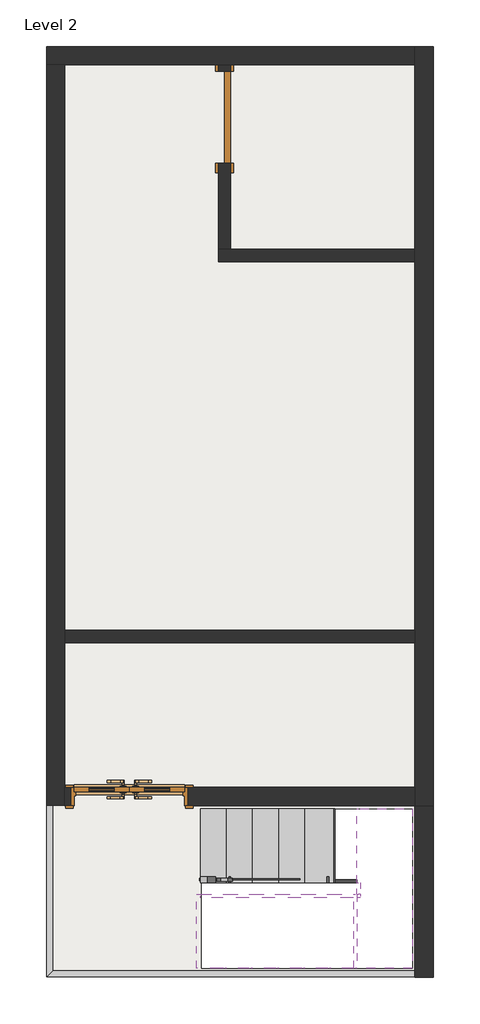
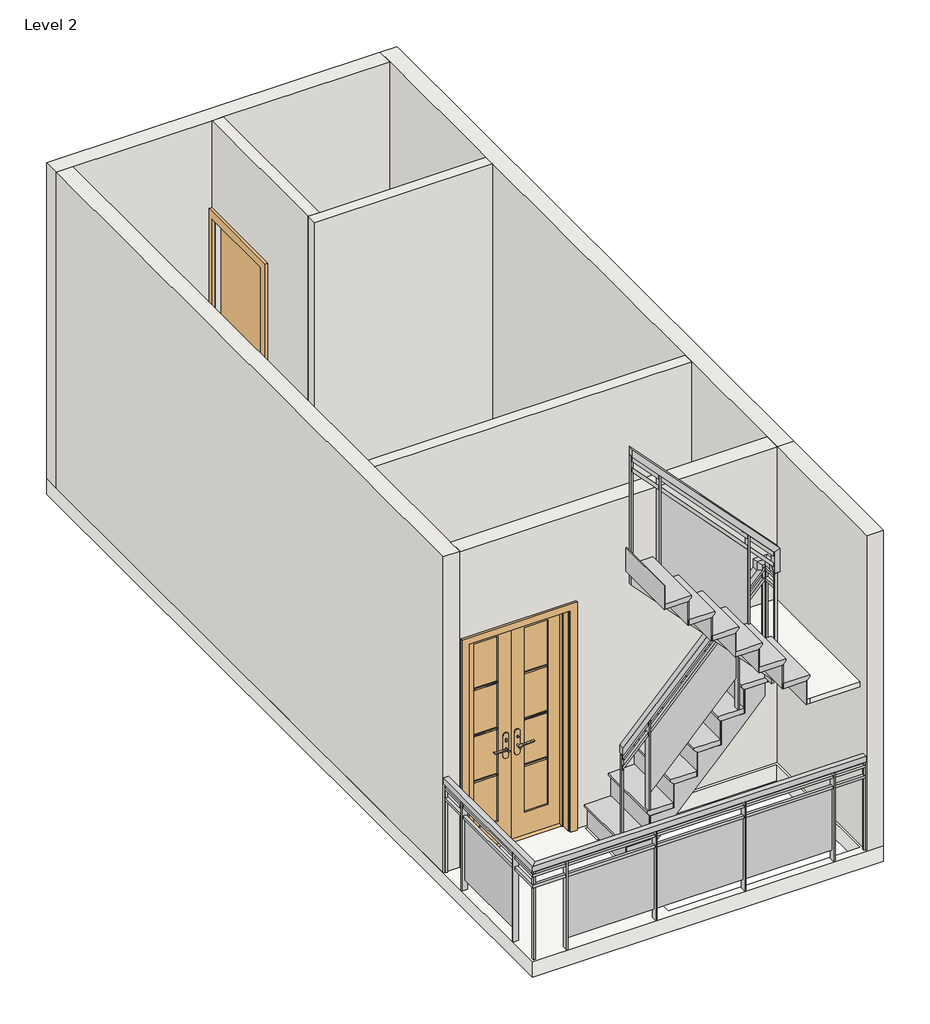
# One storey: 8 walls, 3 members, 2 doors, 2 railings, 2 slabs, 2 stair flights.
"""IFC4 building model written with IfcOpenShell, lengths in millimetres."""

from ifc_helpers import new_model, si_unit, frame, origin, place, context, project, spatial, polyline, outline, extrude, faceted_brep, transform, mapped, element, save
from components import door_665efd91, single_flush_2_5_aa9e95e7, non_monolithic_landing_3bfbdf2e, stair_flight_d5a7a9e1, stair_flight_0dc73603

model = new_model("IFC4")

# Units and contexts
model_context = context("Model", 3, world=origin())
ifc_project = project(units=[si_unit("LENGTHUNIT", "METRE", prefix="MILLI")], contexts=[model_context])

# Site, building, storey
site = spatial("IfcSite", under=ifc_project)
building = spatial("IfcBuilding", under=site)
storey = spatial("IfcBuildingStorey", under=building, Name="Level 2", Elevation=3200.4)

# Doors
placement = place(None, origin())
door_shape = door_665efd91(model_context)
element("IfcDoor", 1, ObjectType="Door-Exterior-Double-Full Glass-Wood_Clad : 60\" x 84\"", at=placement, inside=storey, context=model_context, shape_type="MappedRepresentation", body=[
    mapped(door_shape, transform((-5617.280937, -3133.7029636, 3200.4), x_axis=(1.0, 0.0, 0.0), y_axis=(0.0, 1.0, 0.0), z_axis=(0.0, 0.0, 1.0))),
])
single_flush_2_5_shape = single_flush_2_5_aa9e95e7(model_context)
element("IfcDoor", 2, ObjectType="Single-Flush : 2.5'", at=placement, inside=storey, context=model_context, shape_type="MappedRepresentation", body=[
    mapped(single_flush_2_5_shape, transform((-4829.880937, 2480.8335625, 3200.4), x_axis=(0.0, 1.0, 0.0), y_axis=(-1.0, 0.0, 0.0), z_axis=(0.0, 0.0, 1.0))),
])

# Members
element("IfcMember", 3, ObjectType="Carriage - 2\" Width", at=placement, inside=storey, context=model_context, shape_type="Brep", body=[
    faceted_brep([(-4996.3909298, -3822.6779636, 3200.4), (-4861.0694778, -3822.6779636, 3200.4), (-4861.0694778, -3848.0779636, 3200.4), (-4996.3909298, -3848.0779636, 3200.4), (-3732.7409298, -3822.6779636, 4395.1008155), (-3732.7409298, -3848.0779636, 4395.1008155), (-3916.8909298, -3848.0779636, 4200.1184625), (-4132.7909298, -3848.0779636, 3971.5184625), (-4348.6909298, -3848.0779636, 3742.9184625), (-4564.5909298, -3848.0779636, 3514.3184625), (-4780.4909298, -3848.0779636, 3285.7184625), (-3732.7409298, -3822.6779636, 4521.2), (-4996.3909298, -3822.6779636, 3378.2), (-4780.4909298, -3822.6779636, 3378.2), (-4780.4909298, -3822.6779636, 3606.8), (-4564.5909298, -3822.6779636, 3606.8), (-4564.5909298, -3822.6779636, 3835.4), (-4348.6909298, -3822.6779636, 3835.4), (-4348.6909298, -3822.6779636, 4064.0), (-4132.7909298, -3822.6779636, 4064.0), (-4132.7909298, -3822.6779636, 4292.6), (-3916.8909298, -3822.6779636, 4292.6), (-3916.8909298, -3822.6779636, 4521.2), (-3916.8909298, -3848.0779636, 4521.2), (-3732.7409298, -3848.0779636, 4521.2), (-3916.8909298, -3848.0779636, 4292.6), (-4132.7909298, -3848.0779636, 4292.6), (-4132.7909298, -3848.0779636, 4064.0), (-4348.6909298, -3848.0779636, 4064.0), (-4348.6909298, -3848.0779636, 3835.4), (-4564.5909298, -3848.0779636, 3835.4), (-4564.5909298, -3848.0779636, 3606.8), (-4780.4909298, -3848.0779636, 3606.8), (-4780.4909298, -3848.0779636, 3378.2), (-4996.3909298, -3848.0779636, 3378.2)], [[[0, 1, 2, 3]], [[4, 5, 6, 7, 8, 9, 10, 2, 1]], [[11, 4, 1, 0, 12, 13, 14, 15, 16, 17, 18, 19, 20, 21, 22]], [[22, 23, 24, 11]], [[5, 24, 23, 25, 26, 27, 28, 29, 30, 31, 32, 33, 34, 3, 2, 10, 9, 8, 7, 6]], [[34, 12, 0, 3]], [[12, 34, 33, 13]], [[13, 33, 32, 14]], [[14, 32, 31, 15]], [[15, 31, 30, 16]], [[16, 30, 29, 17]], [[17, 29, 28, 18]], [[18, 28, 27, 19]], [[19, 27, 26, 20]], [[20, 26, 25, 21]], [[21, 25, 23, 22]], [[5, 4, 11, 24]]]),
])
element("IfcMember", 4, ObjectType="Carriage - 2\" Width", at=placement, inside=storey, context=model_context, shape_type="Brep", body=[
    faceted_brep([(-5028.1409298, -3945.3664375, 5995.3008155), (-5028.1409298, -3970.7664375, 5995.3008155), (-5028.1409298, -3970.7664375, 6121.4), (-5028.1409298, -3945.3664375, 6121.4), (-3707.3409298, -3970.7664375, 4596.8066978), (-3707.3409298, -3970.7664375, 4749.8), (-3764.4909298, -3970.7664375, 4749.8), (-3764.4909298, -3970.7664375, 4978.4), (-3980.3909298, -3970.7664375, 4978.4), (-3980.3909298, -3970.7664375, 5207.0), (-4196.2909298, -3970.7664375, 5207.0), (-4196.2909298, -3970.7664375, 5435.6), (-4412.1909298, -3970.7664375, 5435.6), (-4412.1909298, -3970.7664375, 5664.2), (-4628.0909298, -3970.7664375, 5664.2), (-4628.0909298, -3970.7664375, 5892.8), (-4843.9909298, -3970.7664375, 5892.8), (-4843.9909298, -3970.7664375, 6121.4), (-4843.9909298, -3945.3664375, 5800.3184625), (-4628.0909298, -3945.3664375, 5571.7184625), (-4412.1909298, -3945.3664375, 5343.1184625), (-4196.2909298, -3945.3664375, 5114.5184625), (-3980.3909298, -3945.3664375, 4885.9184625), (-3764.4909298, -3945.3664375, 4657.3184625), (-3732.7409298, -3945.3664375, 4623.7008155), (-3707.3409298, -3945.3664375, 4596.8066978), (-4843.9909298, -3945.3664375, 6121.4), (-4843.9909298, -3945.3664375, 5892.8), (-4628.0909298, -3945.3664375, 5892.8), (-4628.0909298, -3945.3664375, 5664.2), (-4412.1909298, -3945.3664375, 5664.2), (-4412.1909298, -3945.3664375, 5435.6), (-4196.2909298, -3945.3664375, 5435.6), (-4196.2909298, -3945.3664375, 5207.0), (-3980.3909298, -3945.3664375, 5207.0), (-3980.3909298, -3945.3664375, 4978.4), (-3764.4909298, -3945.3664375, 4978.4), (-3764.4909298, -3945.3664375, 4749.8), (-3732.7409298, -3945.3664375, 4749.8), (-3707.3409298, -3945.3664375, 4749.8)], [[[0, 1, 2, 3]], [[1, 4, 5, 6, 7, 8, 9, 10, 11, 12, 13, 14, 15, 16, 17, 2]], [[1, 0, 18, 19, 20, 21, 22, 23, 24, 25, 4]], [[0, 3, 26, 27, 28, 29, 30, 31, 32, 33, 34, 35, 36, 37, 38, 39, 25, 24, 23, 22, 21, 20, 19, 18]], [[7, 36, 35, 8]], [[36, 7, 6, 37]], [[9, 34, 33, 10]], [[8, 35, 34, 9]], [[11, 32, 31, 12]], [[10, 33, 32, 11]], [[13, 30, 29, 14]], [[12, 31, 30, 13]], [[15, 28, 27, 16]], [[14, 29, 28, 15]], [[17, 26, 3, 2]], [[16, 27, 26, 17]], [[4, 25, 39, 5]], [[37, 6, 5, 39, 38]]]),
])
element("IfcMember", 5, ObjectType="Carriage - 2\" Width", at=placement, inside=storey, context=model_context, shape_type="SweptSolid", body=[
    extrude(outline(polyline([(-3707.3409298, -3945.3664375), (-3732.7409298, -3945.3664375), (-3732.7409298, -3848.0779636), (-3707.3409298, -3848.0779636), (-3707.3409298, -3945.3664375)])), frame((0.0, 0.0, 4572.0), z_axis=(0.0, 0.0, 1.0), x_axis=(1.0, 0.0, 0.0)), (0.0, 0.0, 1.0), 177.8),
])

# Railings
element("IfcRailing", 6, ObjectType="Glass Panel - Bottom Fill", at=placement, inside=storey, context=model_context, shape_type="SolidModel", body=[
    faceted_brep([(-5028.1409298, -3797.2779636, 4343.4), (-5028.1409298, -3797.2779636, 4269.41477), (-5028.1409298, -3848.0779636, 4269.41477), (-5028.1409298, -3848.0779636, 4343.4), (-3808.9409298, -3797.2779636, 5634.3176471), (-3758.1409298, -3797.2779636, 5614.1206524), (-3758.1409298, -3848.0779636, 5614.1206524), (-3808.9409298, -3848.0779636, 5634.3176471), (-3681.9409298, -3945.3664375, 5715.0), (-3732.7409298, -3945.3664375, 5715.0), (-3732.7409298, -3996.1664375, 5664.2), (-3681.9409298, -3996.1664375, 5664.2), (-3681.9409298, -3924.2779636, 5664.2), (-3681.9409298, -3924.2779636, 5715.0), (-3732.7409298, -3924.2779636, 5664.2), (-3732.7409298, -3924.2779636, 5715.0), (-3808.9409298, -3797.2779636, 5715.0), (-3758.1409298, -3797.2779636, 5664.2), (-3758.1409298, -3848.0779636, 5664.2), (-3808.9409298, -3848.0779636, 5715.0), (-3681.9409298, -3797.2779636, 5715.0), (-3681.9409298, -3797.2779636, 5664.2), (-3732.7409298, -3848.0779636, 5664.2), (-3732.7409298, -3848.0779636, 5715.0)], [[[0, 1, 2, 3]], [[1, 0, 4, 5]], [[2, 1, 5, 6]], [[3, 2, 6, 7]], [[0, 3, 7, 4]], [[8, 9, 10, 11]], [[12, 13, 8, 11]], [[14, 12, 11, 10]], [[15, 14, 10, 9]], [[13, 15, 9, 8]], [[5, 4, 16, 17]], [[6, 5, 17, 18]], [[7, 6, 18, 19]], [[4, 7, 19, 16]], [[17, 16, 20, 21]], [[18, 17, 21, 22]], [[19, 18, 22, 23]], [[16, 19, 23, 20]], [[21, 20, 13, 12]], [[22, 21, 12, 14]], [[23, 22, 14, 15]], [[20, 23, 15, 13]]]),
    faceted_brep([(-3681.9409298, -3996.1664375, 5889.8117647), (-3732.7409298, -3996.1664375, 5869.61477), (-3732.7409298, -3945.3664375, 5869.61477), (-3681.9409298, -3945.3664375, 5889.8117647), (-5028.1409298, -3996.1664375, 7315.2), (-5028.1409298, -3945.3664375, 7315.2), (-5028.1409298, -3945.3664375, 7241.21477), (-5028.1409298, -3996.1664375, 7241.21477)], [[[0, 1, 2, 3]], [[4, 5, 6, 7]], [[1, 0, 4, 7]], [[2, 1, 7, 6]], [[3, 2, 6, 5]], [[0, 3, 5, 4]]]),
    faceted_brep([(-3681.9409298, -3945.3664375, 5715.0), (-3681.9409298, -3996.1664375, 5664.2), (-3732.7409298, -3996.1664375, 5664.2), (-3732.7409298, -3945.3664375, 5715.0), (-3681.9409298, -3945.3664375, 5889.8117647), (-3732.7409298, -3945.3664375, 5869.61477), (-3732.7409298, -3996.1664375, 5869.61477), (-3681.9409298, -3996.1664375, 5889.8117647)], [[[0, 1, 2, 3]], [[4, 5, 6, 7]], [[1, 0, 4, 7]], [[2, 1, 7, 6]], [[3, 2, 6, 5]], [[0, 3, 5, 4]]]),
    faceted_brep([(-5028.1409298, -3835.3779636, 4260.2963075), (-5028.1409298, -3809.9779636, 4260.2963075), (-5028.1409298, -3809.9779636, 4223.3036925), (-5028.1409298, -3835.3779636, 4223.3036925), (-3738.2152202, -3835.3779636, 5626.1), (-3738.2152202, -3809.9779636, 5626.1), (-3727.2666394, -3809.9779636, 5600.7), (-3727.2666394, -3835.3779636, 5600.7), (-3720.0409298, -3835.3779636, 5626.1), (-3694.6409298, -3809.9779636, 5626.1), (-3694.6409298, -3809.9779636, 5600.7), (-3720.0409298, -3835.3779636, 5600.7), (-3720.0409298, -3958.0664375, 5626.1), (-3720.0409298, -3958.0664375, 5600.7), (-3694.6409298, -3958.0664375, 5600.7), (-3694.6409298, -3958.0664375, 5626.1)], [[[0, 1, 2, 3]], [[1, 0, 4, 5]], [[2, 1, 5, 6]], [[3, 2, 6, 7]], [[0, 3, 7, 4]], [[5, 4, 8, 9]], [[6, 5, 9, 10]], [[7, 6, 10, 11]], [[4, 7, 11, 8]], [[12, 13, 14, 15]], [[9, 8, 12, 15]], [[10, 9, 15, 14]], [[11, 10, 14, 13]], [[8, 11, 13, 12]]]),
    faceted_brep([(-3694.6409298, -3958.0664375, 5820.155131), (-3694.6409298, -3983.4664375, 5820.155131), (-3694.6409298, -3983.4664375, 5783.162516), (-3694.6409298, -3958.0664375, 5783.162516), (-5028.1409298, -3958.0664375, 7232.0963075), (-5028.1409298, -3958.0664375, 7195.1036925), (-5028.1409298, -3983.4664375, 7195.1036925), (-5028.1409298, -3983.4664375, 7232.0963075)], [[[0, 1, 2, 3]], [[4, 5, 6, 7]], [[1, 0, 4, 7]], [[2, 1, 7, 6]], [[3, 2, 6, 5]], [[0, 3, 5, 4]]]),
    faceted_brep([(-5028.1409298, -3835.3779636, 4158.6963075), (-5028.1409298, -3809.9779636, 4158.6963075), (-5028.1409298, -3809.9779636, 4121.7036925), (-5028.1409298, -3835.3779636, 4121.7036925), (-3738.2152202, -3835.3779636, 5524.5), (-3738.2152202, -3809.9779636, 5524.5), (-3727.2666394, -3809.9779636, 5499.1), (-3727.2666394, -3835.3779636, 5499.1), (-3720.0409298, -3835.3779636, 5524.5), (-3694.6409298, -3809.9779636, 5524.5), (-3694.6409298, -3809.9779636, 5499.1), (-3720.0409298, -3835.3779636, 5499.1), (-3720.0409298, -3958.0664375, 5524.5), (-3720.0409298, -3958.0664375, 5499.1), (-3694.6409298, -3958.0664375, 5499.1), (-3694.6409298, -3958.0664375, 5524.5)], [[[0, 1, 2, 3]], [[1, 0, 4, 5]], [[2, 1, 5, 6]], [[3, 2, 6, 7]], [[0, 3, 7, 4]], [[5, 4, 8, 9]], [[6, 5, 9, 10]], [[7, 6, 10, 11]], [[4, 7, 11, 8]], [[12, 13, 14, 15]], [[9, 8, 12, 15]], [[10, 9, 15, 14]], [[11, 10, 14, 13]], [[8, 11, 13, 12]]]),
    faceted_brep([(-3694.6409298, -3958.0664375, 5718.555131), (-3694.6409298, -3983.4664375, 5718.555131), (-3694.6409298, -3983.4664375, 5681.562516), (-3694.6409298, -3958.0664375, 5681.562516), (-5028.1409298, -3958.0664375, 7130.4963075), (-5028.1409298, -3958.0664375, 7093.5036925), (-5028.1409298, -3983.4664375, 7093.5036925), (-5028.1409298, -3983.4664375, 7130.4963075)], [[[0, 1, 2, 3]], [[4, 5, 6, 7]], [[1, 0, 4, 7]], [[2, 1, 7, 6]], [[3, 2, 6, 5]], [[0, 3, 5, 4]]]),
    extrude(outline(polyline([(6965.5500641, -4767.7909298), (6978.997123, -4780.4909298), (5943.6, -4780.4909298), (5943.6, -4767.7909298), (6965.5500641, -4767.7909298)])), frame((0.0, -3996.1664375, 0.0), z_axis=(0.0, 1.0, 0.0), x_axis=(0.0, 0.0, 1.0)), (0.0, 0.0, 1.0), 50.8),
    extrude(outline(polyline([(5157.6941176, -3961.3409298), (5963.9507513, -3961.3409298), (6824.562516, -4774.1409298), (6018.3058824, -4774.1409298), (5157.6941176, -3961.3409298)])), frame((0.0, -3977.3015945, 0.0), z_axis=(0.0, 1.0, 0.0), x_axis=(0.0, 0.0, 1.0)), (0.0, 0.0, 1.0), 6.35),
    extrude(outline(polyline([(6104.9382994, -3954.9909298), (6118.3853582, -3967.6909298), (5257.8, -3967.6909298), (5257.8, -3954.9909298), (6104.9382994, -3954.9909298)])), frame((0.0, -3996.1664375, 0.0), z_axis=(0.0, 1.0, 0.0), x_axis=(0.0, 0.0, 1.0)), (0.0, 0.0, 1.0), 50.8),
    extrude(outline(polyline([(5392.2441818, -3967.6909298), (5378.797123, -3980.3909298), (4343.4, -3980.3909298), (4343.4, -3967.6909298), (5392.2441818, -3967.6909298)])), frame((0.0, -3848.0779636, 0.0), z_axis=(0.0, 1.0, 0.0), x_axis=(0.0, 0.0, 1.0)), (0.0, 0.0, 1.0), 50.8),
    extrude(outline(polyline([(3786.0941176, -4786.8409298), (4646.7058824, -3974.0409298), (5237.8095749, -3974.0409298), (4377.1978102, -4786.8409298), (3786.0941176, -4786.8409298)])), frame((0.0, -3822.4928066, 0.0), z_axis=(0.0, 1.0, 0.0), x_axis=(0.0, 0.0, 1.0)), (0.0, 0.0, 1.0), 6.35),
    extrude(outline(polyline([(4531.6324171, -4780.4909298), (4518.1853582, -4793.1909298), (3657.6, -4793.1909298), (3657.6, -4780.4909298), (4531.6324171, -4780.4909298)])), frame((0.0, -3848.0779636, 0.0), z_axis=(0.0, 1.0, 0.0), x_axis=(0.0, 0.0, 1.0)), (0.0, 0.0, 1.0), 50.8),
    extrude(outline(polyline([(-3697.8159298, -3961.2414375), (-3697.8159298, -3980.2914375), (-3716.8659298, -3980.2914375), (-3716.8659298, -3961.2414375), (-3697.8159298, -3961.2414375)])), frame((0.0, 0.0, 4800.6), z_axis=(0.0, 0.0, 1.0), x_axis=(1.0, 0.0, 0.0)), (0.0, 0.0, 1.0), 863.6),
    extrude(outline(polyline([(-3716.8659298, -3832.2029636), (-3716.8659298, -3813.1529636), (-3697.8159298, -3813.1529636), (-3697.8159298, -3832.2029636), (-3716.8659298, -3832.2029636)])), frame((0.0, 0.0, 4800.6), z_axis=(0.0, 0.0, 1.0), x_axis=(1.0, 0.0, 0.0)), (0.0, 0.0, 1.0), 863.6),
    extrude(outline(polyline([(-3742.2659298, -3832.2029636), (-3742.2659298, -3813.1529636), (-3723.2159298, -3813.1529636), (-3723.2159298, -3832.2029636), (-3742.2659298, -3832.2029636)])), frame((0.0, 0.0, 4800.6), z_axis=(0.0, 0.0, 1.0), x_axis=(1.0, 0.0, 0.0)), (0.0, 0.0, 1.0), 863.6),
    extrude(outline(polyline([(7227.7677112, -5015.4409298), (7247.9382994, -5034.4909298), (6172.2, -5034.4909298), (6172.2, -5015.4409298), (7227.7677112, -5015.4409298)])), frame((0.0, -3980.2914375, 0.0), z_axis=(0.0, 1.0, 0.0), x_axis=(0.0, 0.0, 1.0)), (0.0, 0.0, 1.0), 19.05),
    extrude(outline(polyline([(4282.8618288, -5015.4409298), (4262.6912406, -5034.4909298), (3429.0, -5034.4909298), (3429.0, -5015.4409298), (4282.8618288, -5015.4409298)])), frame((0.0, -3832.2029636, 0.0), z_axis=(0.0, 1.0, 0.0), x_axis=(0.0, 0.0, 1.0)), (0.0, 0.0, 1.0), 19.05),
])
element("IfcRailing", 7, ObjectType="Glass Panel - Bottom Fill", at=placement, inside=storey, context=model_context, shape_type="SolidModel", body=[
    faceted_brep([(-6252.280937, -3208.7664375, 4114.8), (-6252.280937, -3208.7664375, 4064.0), (-6303.080937, -3208.7664375, 4064.0), (-6303.080937, -3208.7664375, 4114.8), (-6252.280937, -4574.0164375, 4114.8), (-6252.280937, -4574.0164375, 4064.0), (-6303.080937, -4624.8164375, 4064.0), (-6303.080937, -4624.8164375, 4114.8), (-3255.080937, -4574.0164375, 4114.8), (-3255.080937, -4624.8164375, 4114.8), (-3255.080937, -4624.8164375, 4064.0), (-3255.080937, -4574.0164375, 4064.0)], [[[0, 1, 2, 3]], [[1, 0, 4, 5]], [[2, 1, 5, 6]], [[3, 2, 6, 7]], [[0, 3, 7, 4]], [[8, 9, 10, 11]], [[5, 4, 8, 11]], [[6, 5, 11, 10]], [[7, 6, 10, 9]], [[4, 7, 9, 8]]]),
    faceted_brep([(-6290.380937, -3208.7664375, 4025.9), (-6264.980937, -3208.7664375, 4025.9), (-6264.980937, -3208.7664375, 4000.5), (-6290.380937, -3208.7664375, 4000.5), (-6290.380937, -4612.1164375, 4025.9), (-6264.980937, -4586.7164375, 4025.9), (-6264.980937, -4586.7164375, 4000.5), (-6290.380937, -4612.1164375, 4000.5), (-3255.080937, -4612.1164375, 4025.9), (-3255.080937, -4612.1164375, 4000.5), (-3255.080937, -4586.7164375, 4000.5), (-3255.080937, -4586.7164375, 4025.9)], [[[0, 1, 2, 3]], [[1, 0, 4, 5]], [[2, 1, 5, 6]], [[3, 2, 6, 7]], [[0, 3, 7, 4]], [[8, 9, 10, 11]], [[5, 4, 8, 11]], [[6, 5, 11, 10]], [[7, 6, 10, 9]], [[4, 7, 9, 8]]]),
    faceted_brep([(-6290.380937, -3208.7664375, 3924.3), (-6264.980937, -3208.7664375, 3924.3), (-6264.980937, -3208.7664375, 3898.9), (-6290.380937, -3208.7664375, 3898.9), (-6290.380937, -4612.1164375, 3924.3), (-6264.980937, -4586.7164375, 3924.3), (-6264.980937, -4586.7164375, 3898.9), (-6290.380937, -4612.1164375, 3898.9), (-3255.080937, -4612.1164375, 3924.3), (-3255.080937, -4612.1164375, 3898.9), (-3255.080937, -4586.7164375, 3898.9), (-3255.080937, -4586.7164375, 3924.3)], [[[0, 1, 2, 3]], [[1, 0, 4, 5]], [[2, 1, 5, 6]], [[3, 2, 6, 7]], [[0, 3, 7, 4]], [[8, 9, 10, 11]], [[5, 4, 8, 11]], [[6, 5, 11, 10]], [[7, 6, 10, 9]], [[4, 7, 9, 8]]]),
    extrude(outline(polyline([(-3553.530937, -4624.8164375), (-3553.530937, -4574.0164375), (-3540.830937, -4574.0164375), (-3540.830937, -4624.8164375), (-3553.530937, -4624.8164375)])), frame((0.0, 0.0, 3200.4), z_axis=(0.0, 0.0, 1.0), x_axis=(1.0, 0.0, 0.0)), (0.0, 0.0, 1.0), 863.6),
    extrude(outline(polyline([(-4359.980937, -4592.8812805), (-3547.180937, -4592.8812805), (-3547.180937, -4599.2312805), (-4359.980937, -4599.2312805), (-4359.980937, -4592.8812805)])), frame((0.0, 0.0, 3302.0), z_axis=(0.0, 0.0, 1.0), x_axis=(1.0, 0.0, 0.0)), (0.0, 0.0, 1.0), 596.9),
    extrude(outline(polyline([(-4366.330937, -4624.8164375), (-4366.330937, -4574.0164375), (-4353.630937, -4574.0164375), (-4353.630937, -4624.8164375), (-4366.330937, -4624.8164375)])), frame((0.0, 0.0, 3200.4), z_axis=(0.0, 0.0, 1.0), x_axis=(1.0, 0.0, 0.0)), (0.0, 0.0, 1.0), 863.6),
    extrude(outline(polyline([(-5172.780937, -4592.8812805), (-4359.980937, -4592.8812805), (-4359.980937, -4599.2312805), (-5172.780937, -4599.2312805), (-5172.780937, -4592.8812805)])), frame((0.0, 0.0, 3302.0), z_axis=(0.0, 0.0, 1.0), x_axis=(1.0, 0.0, 0.0)), (0.0, 0.0, 1.0), 596.9),
    extrude(outline(polyline([(-5179.130937, -4624.8164375), (-5179.130937, -4574.0164375), (-5166.430937, -4574.0164375), (-5166.430937, -4624.8164375), (-5179.130937, -4624.8164375)])), frame((0.0, 0.0, 3200.4), z_axis=(0.0, 0.0, 1.0), x_axis=(1.0, 0.0, 0.0)), (0.0, 0.0, 1.0), 863.6),
    extrude(outline(polyline([(-5985.580937, -4592.8812805), (-5172.780937, -4592.8812805), (-5172.780937, -4599.2312805), (-5985.580937, -4599.2312805), (-5985.580937, -4592.8812805)])), frame((0.0, 0.0, 3302.0), z_axis=(0.0, 0.0, 1.0), x_axis=(1.0, 0.0, 0.0)), (0.0, 0.0, 1.0), 596.9),
    extrude(outline(polyline([(-5991.930937, -4624.8164375), (-5991.930937, -4574.0164375), (-5979.230937, -4574.0164375), (-5979.230937, -4624.8164375), (-5991.930937, -4624.8164375)])), frame((0.0, 0.0, 3200.4), z_axis=(0.0, 0.0, 1.0), x_axis=(1.0, 0.0, 0.0)), (0.0, 0.0, 1.0), 863.6),
    extrude(outline(polyline([(-6303.080937, -4304.1414375), (-6252.280937, -4304.1414375), (-6252.280937, -4316.8414375), (-6303.080937, -4316.8414375), (-6303.080937, -4304.1414375)])), frame((0.0, 0.0, 3200.4), z_axis=(0.0, 0.0, 1.0), x_axis=(1.0, 0.0, 0.0)), (0.0, 0.0, 1.0), 863.6),
    extrude(outline(polyline([(-6271.14578, -3497.6914375), (-6271.14578, -4310.4914375), (-6277.49578, -4310.4914375), (-6277.49578, -3497.6914375), (-6271.14578, -3497.6914375)])), frame((0.0, 0.0, 3302.0), z_axis=(0.0, 0.0, 1.0), x_axis=(1.0, 0.0, 0.0)), (0.0, 0.0, 1.0), 596.9),
    extrude(outline(polyline([(-6303.080937, -3491.3414375), (-6252.280937, -3491.3414375), (-6252.280937, -3504.0414375), (-6303.080937, -3504.0414375), (-6303.080937, -3491.3414375)])), frame((0.0, 0.0, 3200.4), z_axis=(0.0, 0.0, 1.0), x_axis=(1.0, 0.0, 0.0)), (0.0, 0.0, 1.0), 863.6),
    extrude(outline(polyline([(-6287.205937, -4589.8914375), (-6268.155937, -4589.8914375), (-6268.155937, -4608.9414375), (-6287.205937, -4608.9414375), (-6287.205937, -4589.8914375)])), frame((0.0, 0.0, 3200.4), z_axis=(0.0, 0.0, 1.0), x_axis=(1.0, 0.0, 0.0)), (0.0, 0.0, 1.0), 863.6),
    extrude(outline(polyline([(-3267.780937, -4608.9414375), (-3267.780937, -4589.8914375), (-3248.730937, -4589.8914375), (-3248.730937, -4608.9414375), (-3267.780937, -4608.9414375)])), frame((0.0, 0.0, 3200.4), z_axis=(0.0, 0.0, 1.0), x_axis=(1.0, 0.0, 0.0)), (0.0, 0.0, 1.0), 863.6),
    extrude(outline(polyline([(-6287.205937, -3202.4164375), (-6268.155937, -3202.4164375), (-6268.155937, -3221.4664375), (-6287.205937, -3221.4664375), (-6287.205937, -3202.4164375)])), frame((0.0, 0.0, 3200.4), z_axis=(0.0, 0.0, 1.0), x_axis=(1.0, 0.0, 0.0)), (0.0, 0.0, 1.0), 863.6),
])

# Slabs
element("IfcSlab", 8, ObjectType="6\"", at=placement, inside=storey, context=model_context, shape_type="SweptSolid", body=[
    extrude(outline(polyline([(-3102.680937, 3065.0335625), (-3102.680937, -4624.8164375), (-6303.080937, -4624.8164375), (-6303.080937, 3065.0335625), (-3102.680937, 3065.0335625)]), holes=[polyline([(-5021.7909298, -3238.4779636), (-5021.7909298, -4554.9664375), (-3275.5409298, -4554.9664375), (-3275.5409298, -3238.4779636), (-5021.7909298, -3238.4779636)])]), frame((0.0, 0.0, 3048.0), z_axis=(0.0, 0.0, 1.0), x_axis=(1.0, 0.0, 0.0)), (0.0, 0.0, 1.0), 152.4),
])
non_monolithic_landing_shape = non_monolithic_landing_3bfbdf2e(model_context)
element("IfcSlab", 9, ObjectType="Non-Monolithic Landing", at=placement, inside=storey, context=model_context, shape_type="MappedRepresentation", body=[
    mapped(non_monolithic_landing_shape, transform((0.0, 0.0, 0.0), x_axis=(1.0, 0.0, 0.0), y_axis=(0.0, 1.0, 0.0), z_axis=(0.0, 0.0, 1.0))),
])

# Stair flights
stair_flight_shape = stair_flight_d5a7a9e1(model_context)
element("IfcStairFlight", 10, ObjectType="2\" Tread 1\" Nosing 1/4\" Riser", at=placement, inside=storey, context=model_context, shape_type="MappedRepresentation", body=[
    mapped(stair_flight_shape, transform((0.0, 0.0, 0.0), x_axis=(1.0, 0.0, 0.0), y_axis=(0.0, 1.0, 0.0), z_axis=(0.0, 0.0, 1.0))),
])
stair_flight_2_shape = stair_flight_0dc73603(model_context)
element("IfcStairFlight", 11, ObjectType="2\" Tread 1\" Nosing 1/4\" Riser", at=placement, inside=storey, context=model_context, shape_type="MappedRepresentation", body=[
    mapped(stair_flight_2_shape, transform((0.0, 0.0, 0.0), x_axis=(1.0, 0.0, 0.0), y_axis=(0.0, 1.0, 0.0), z_axis=(0.0, 0.0, 1.0))),
])

# Walls
element("IfcWall", 12, ObjectType="4\"", at=placement, inside=storey, context=model_context, shape_type="Brep", body=[
    faceted_brep([(-3255.080937, 1388.6335625, 3200.4), (-4779.080937, 1388.6335625, 3200.4), (-4880.680937, 1388.6335625, 3200.4), (-4880.680937, 1388.6335625, 6248.4), (-4779.080937, 1388.6335625, 6248.4), (-3255.080937, 1388.6335625, 6248.4), (-3255.080937, 1287.0335625, 3200.4), (-3255.080937, 1287.0335625, 6248.4), (-4880.680937, 1287.0335625, 6248.4), (-4880.680937, 1287.0335625, 3200.4)], [[[0, 1, 2, 3, 4, 5]], [[6, 7, 8, 9]], [[2, 1, 0, 6, 9]], [[5, 4, 3, 8, 7]], [[0, 5, 7, 6]], [[3, 2, 9, 8]]]),
])
element("IfcWall", 13, ObjectType="4\"", at=placement, inside=storey, context=model_context, shape_type="SweptSolid", body=[
    extrude(outline(polyline([(2912.6335625, 3200.4), (2861.8335625, 3200.4), (2861.8335625, 5334.0), (2099.8335625, 5334.0), (2099.8335625, 3200.4), (1388.6335625, 3200.4), (1388.6335625, 6248.4), (2912.6335625, 6248.4), (2912.6335625, 3200.4)])), frame((-4880.680937, 0.0, 0.0), z_axis=(1.0, 0.0, 0.0), x_axis=(0.0, 1.0, 0.0)), (0.0, 0.0, 1.0), 101.6),
])
element("IfcWall", 14, ObjectType="4\"", at=placement, inside=storey, context=model_context, shape_type="SweptSolid", body=[
    extrude(outline(polyline([(-6150.680937, -1760.9664375), (-3255.080937, -1760.9664375), (-3255.080937, -1862.5664375), (-6150.680937, -1862.5664375), (-6150.680937, -1760.9664375)])), frame((0.0, 0.0, 3200.4), z_axis=(0.0, 0.0, 1.0), x_axis=(1.0, 0.0, 0.0)), (0.0, 0.0, 1.0), 3048.0),
])
element("IfcWall", 15, ObjectType="6\"", at=placement, inside=storey, context=model_context, shape_type="Brep", body=[
    faceted_brep([(-6303.080937, 2912.6335625, 3200.4), (-6150.680937, 2912.6335625, 3200.4), (-4880.680937, 2912.6335625, 3200.4), (-4779.080937, 2912.6335625, 3200.4), (-3255.080937, 2912.6335625, 3200.4), (-3255.080937, 2912.6335625, 6248.4), (-4779.080937, 2912.6335625, 6248.4), (-4880.680937, 2912.6335625, 6248.4), (-6150.680937, 2912.6335625, 6248.4), (-6303.080937, 2912.6335625, 6248.4), (-6303.080937, 3065.0335625, 3200.4), (-6303.080937, 3065.0335625, 6248.4), (-3255.080937, 3065.0335625, 6248.4), (-3255.080937, 3065.0335625, 3200.4)], [[[0, 1, 2, 3, 4, 5, 6, 7, 8, 9]], [[10, 11, 12, 13]], [[4, 3, 2, 1, 0, 10, 13]], [[9, 8, 7, 6, 5, 12, 11]], [[0, 9, 11, 10]], [[5, 4, 13, 12]]]),
])
element("IfcWall", 16, ObjectType="6\"", at=placement, inside=storey, context=model_context, shape_type="Brep", body=[
    faceted_brep([(-3255.080937, 3065.0335625, 3200.4), (-3255.080937, 2912.6335625, 3200.4), (-3255.080937, 1388.6335625, 3200.4), (-3255.080937, 1287.0335625, 3200.4), (-3255.080937, -1760.9664375, 3200.4), (-3255.080937, -1862.5664375, 3200.4), (-3255.080937, -3060.6779636, 3200.4), (-3255.080937, -3213.0779636, 3200.4), (-3255.080937, -3215.1164375, 3200.4), (-3255.080937, -3215.1164375, 6248.4), (-3255.080937, -3213.0779636, 6248.4), (-3255.080937, -3060.6779636, 6248.4), (-3255.080937, -1862.5664375, 6248.4), (-3255.080937, -1760.9664375, 6248.4), (-3255.080937, 1287.0335625, 6248.4), (-3255.080937, 1388.6335625, 6248.4), (-3255.080937, 2912.6335625, 6248.4), (-3255.080937, 3065.0335625, 6248.4), (-3102.680937, 3065.0335625, 3200.4), (-3102.680937, 3065.0335625, 6248.4), (-3102.680937, -3215.1164375, 6248.4), (-3102.680937, -3215.1164375, 3200.4)], [[[0, 1, 2, 3, 4, 5, 6, 7, 8, 9, 10, 11, 12, 13, 14, 15, 16, 17]], [[18, 19, 20, 21]], [[8, 7, 6, 5, 4, 3, 2, 1, 0, 18, 21]], [[9, 8, 21, 20]], [[17, 16, 15, 14, 13, 12, 11, 10, 9, 20, 19]], [[0, 17, 19, 18]]]),
])
element("IfcWall", 17, ObjectType="6\"", at=placement, inside=storey, context=model_context, shape_type="Brep", body=[
    faceted_brep([(-6150.680937, -3060.6779636, 6248.4), (-3255.080937, -3060.6779636, 6248.4), (-3255.080937, -3060.6779636, 3200.4), (-5134.680937, -3060.6779636, 3200.4), (-5134.680937, -3060.6779636, 5359.4), (-6099.880937, -3060.6779636, 5359.4), (-6099.880937, -3060.6779636, 3200.4), (-6150.680937, -3060.6779636, 3200.4), (-3255.080937, -3213.0779636, 6248.4), (-6150.680937, -3213.0779636, 6248.4), (-6150.680937, -3213.0779636, 3200.4), (-6099.880937, -3213.0779636, 3200.4), (-6099.880937, -3213.0779636, 5359.4), (-5134.680937, -3213.0779636, 5359.4), (-5134.680937, -3213.0779636, 3200.4), (-3255.080937, -3213.0779636, 3200.4), (-6150.680937, -3208.7664375, 3200.4), (-6150.680937, -3208.7664375, 6248.4)], [[[0, 1, 2, 3, 4, 5, 6, 7]], [[8, 9, 10, 11, 12, 13, 14, 15]], [[10, 16, 7, 6, 11]], [[2, 15, 14, 3]], [[1, 0, 17, 9, 8]], [[0, 7, 16, 10, 9, 17]], [[2, 1, 8, 15]], [[13, 4, 3, 14]], [[4, 13, 12, 5]], [[5, 12, 11, 6]]]),
])
element("IfcWall", 18, ObjectType="6\"", at=placement, inside=storey, context=model_context, shape_type="Brep", body=[
    faceted_brep([(-6150.680937, -3208.7664375, 3200.4), (-6150.680937, -3060.6779636, 3200.4), (-6150.680937, -1862.5664375, 3200.4), (-6150.680937, -1760.9664375, 3200.4), (-6150.680937, 2912.6335625, 3200.4), (-6150.680937, 2912.6335625, 6248.4), (-6150.680937, -1760.9664375, 6248.4), (-6150.680937, -1862.5664375, 6248.4), (-6150.680937, -3060.6779636, 6248.4), (-6150.680937, -3208.7664375, 6248.4), (-6303.080937, -3208.7664375, 3200.4), (-6303.080937, -3208.7664375, 6248.4), (-6303.080937, 2912.6335625, 6248.4), (-6303.080937, 2912.6335625, 3200.4)], [[[0, 1, 2, 3, 4, 5, 6, 7, 8, 9]], [[10, 11, 12, 13]], [[4, 3, 2, 1, 0, 10, 13]], [[9, 8, 7, 6, 5, 12, 11]], [[0, 9, 11, 10]], [[5, 4, 13, 12]]]),
])
element("IfcWall", 19, ObjectType="6\"", at=placement, inside=storey, context=model_context, shape_type="SweptSolid", body=[
    extrude(outline(polyline([(-3255.080937, -4631.1664375), (-3255.080937, -3215.1164375), (-3102.680937, -3215.1164375), (-3102.680937, -4631.1664375), (-3255.080937, -4631.1664375)])), frame((0.0, 0.0, 3200.4), z_axis=(0.0, 0.0, 1.0), x_axis=(1.0, 0.0, 0.0)), (0.0, 0.0, 1.0), 3048.0),
])

save(model, "model.ifc")

# Revit data of these elements
# Type "Door-Exterior-Double-Full Glass-Wood_Clad : 60\" x 84\""
#   Type Mark = "8"
#   Assembly Code = "B2030100"
#   Analytic Construction = "French door, wood frame with double glass"
#   Top Rail = 0' - 4 11/16"
#   Threshold Offset [instance default] = 0' - 0 1/2"
#   Thickness = 0' - 1 3/8"
#   Thermal Resistance (R) = 1.9158 (h·ft²·°F)/BTU
#   Swing Angle [instance default] = 90.00°
#   Stiles = 0' - 4 3/4"
#   Rough Width = 3' - 2"
#   Rough Height = 7' - 1"
#   Panel Width = 1' - 6"
#   Door Offset [instance default] = 0' - 0"
#   Height = 7' - 0"
#   Width = 3' - 0"
#   Heat Transfer Coefficient (U) = 0.5220 BTU/(h·ft²·°F)
#   Bottom Rail = 0' - 9 1/8"
#   Exterior Trim [instance default] = yes
#   Threshold [instance default] = yes
#   Show Grill [instance default] = yes
#   Function = 1
#   Trim Material = Cherry
#   Threshold Material = Cherry
#   Panel Material = Cherry
#   Glazing = Glass
#   Frame Material = Cherry
#   Door Handle Material = Aluminum
#   Visual Light Transmittance = 0
#   Solar Heat Gain Coefficient = 0
#   Wall Closure = (empty or 0)
#   Construction Type = (empty or 0)
# Type "Single-Flush : 2.5'"
#   Type Mark = "9"
#   Construction Type Id = "MDOOR"
#   Assembly Code = "C1020"
#   Analytic Construction = "Metal"
#   Thickness = 0' - 2"
#   Heat Transfer Coefficient (U) = 0.651978 BTU/(h·ft²·°F)
#   Height = 7' - 0"
#   Trim Projection Ext = 0' - 1"
#   Trim Projection Int = 0' - 1"
#   Trim Width = 0' - 3"
#   Width = 2' - 6"
#   Define Thermal Properties by = 1
#   Door Material = Door - Panel
#   Frame Material = Door - Frame
#   Visual Light Transmittance = 0
#   Solar Heat Gain Coefficient = 0
#   Function = (empty or 0)
#   Wall Closure = (empty or 0)
# Type "Glass Panel - Bottom Fill"
#   Assembly Code = "C2010400"
#   built-in parameter 1008612 = 0.0416667 (stored number, unit not read)
#   built-in parameter 1008611 = 0.0416667 (stored number, unit not read)
#   built-in parameter 1008609 = 0.333333 (stored number, unit not read)
#   built-in parameter 1008604 = 0.166667 (stored number, unit not read)
#   built-in parameter 1008603 = 0.166667 (stored number, unit not read)
#   Railing Height = 3' - 0"
#   built-in parameter 1008630 = 2
#   built-in parameter 1008610 = 2
#   built-in parameter 1008618 = Baluster - Square : 3/4"
# Type "6\""
#   Assembly Code = "B1010"
#   Function = 0
#   Layers, outside or top first: 0' - 6" no material (function 1)
# Type "4\""
#   Assembly Code = "B2010"
#   Layers, outside or top first: 0' - 4" no material (function 1)
# Type "6\""
#   Assembly Code = "B2010"
#   Layers, outside or top first: 0' - 6" no material (function 1)
# Element 1 (IfcDoor, "Door-Exterior-Double-Full Glass-Wood_Clad : 60\" x 84\"")
#   Threshold Offset = 0' - 0 1/2"
#   Swing Angle = 90.00°
#   Door Offset = 0' - 0"
#   Threshold = yes
#   Show Grill = yes
#   Exterior Trim = yes
#   Phase Created = New Construction
#   Materials on its faces: "Cherry", "Aluminum", "Glass"
# Element 2 (IfcDoor, "Single-Flush : 2.5'")
#   Phase Created = New Construction
#   Materials on its faces: "Door - Frame", "Door - Panel"
# Elements 3, 4, 5 (IfcMember, "Carriage - 2\" Width")
#   Phase Created = New Construction
# Elements 6, 7 (IfcRailing, "Glass Panel - Bottom Fill")
#   Phase Created = New Construction
#   Materials on its faces: "Glass"
# Element 8 (IfcSlab, "6\"")
#   Height Offset From Level = 0' - 0"
#   Phase Created = New Construction
#   Materials on its faces: "Default Floor"
# Element 9 (IfcSlab, "Non-Monolithic Landing")
#   Phase Created = New Construction
# Elements 10, 11 (IfcStairFlight, "2\" Tread 1\" Nosing 1/4\" Riser")
#   Phase Created = New Construction
# Elements 12, 13, 14 (IfcWall, "4\"")
#   Top Offset = 0' - 0"
#   Base Offset = 0' - 0"
#   Unconnected Height = 10' - 0"
#   wall height = 10' - 0"
#   Phase Created = New Construction
#   Base Constraint = Level 2
#   Materials on its faces: "Default Wall"
# Elements 15, 16, 17, 18, 19 (IfcWall, "6\"")
#   Top Offset = 0' - 0"
#   Base Offset = 0' - 0"
#   Unconnected Height = 10' - 0"
#   wall height = 10' - 0"
#   Phase Created = New Construction
#   Base Constraint = Level 2
#   Materials on its faces: "Default Wall"
# Materials
#   "Cherry": class "Wood", colour RGB 226 177 128, transparency 0, Description = "Prunus Serotina", Cost = 0
#   "Glass": class "Glass", colour RGB 0 128 192, transparency 0.75, Description = "Soda Lime Glass", Cost = 0
#   "Aluminum": class "Metal", colour RGB 247 247 247, transparency 0, Description = "Aluminum 6061", Cost = 0
#   "Door - Panel": class "Wood", colour RGB 210 159 95, transparency 0
#   "Door - Frame": colour RGB 118 70 51, transparency 0
#   "Default Floor": colour RGB 128 128 128, transparency 0
#   "Default Wall": colour RGB 128 128 128, transparency 0
